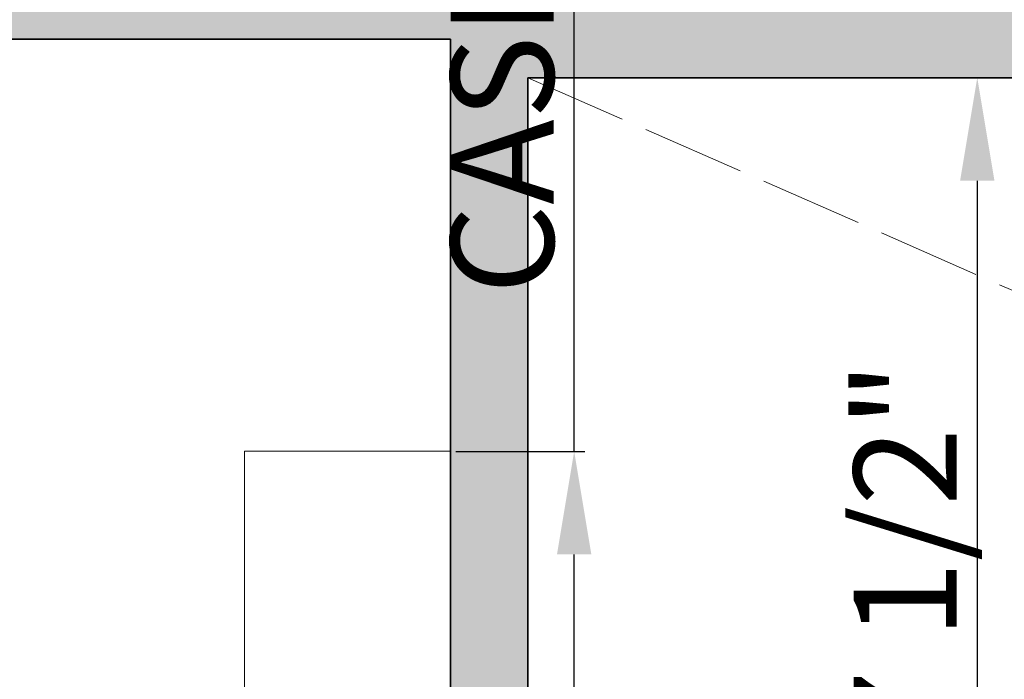
# Model space of a CAD drawing. Units: inches. Extents: x 2083 to 3317, y 1141 to 2115.
# Tile 87 of 256: x 2486 to 2600, y 1342 to 1419. Entities that reach past the tile are written whole.
import ezdxf

# ---------------------------------------------------------------- set-up
doc = ezdxf.new("R2010")
doc.units = ezdxf.units.IN
doc.linetypes.add('ACAD_ISO02W100', pattern=[15, 12, -3])
for name, color, linetype, lineweight in [('A-ANNO-DIMS', 2, 'Continuous', 18), ('A-FLOR-CASE', 8, 'Continuous', 18), ('A-FLOR-OPEN', 8, 'ACAD_ISO02W100', 13), ('A-WALL', 7, 'Continuous', 35)]:
    doc.layers.add(name, color=color, linetype=linetype, lineweight=lineweight)
doc.layers.add('A-WALL-PATT', color=251, linetype='Continuous', lineweight=13, true_color=0x636466)
doc.styles.get("Standard").update_dxf_attribs({"font": 'arial.ttf'})
doc.dimstyles.new('ISO-25', dxfattribs={"dimtxt": 12, "dimasz": 12, "dimexe": 1.25, "dimexo": 0.625, "dimtad": 1, "dimlunit": 3, "dimtxsty": 'Standard', "dimcen": 2.5, "dimadec": 0, "dimazin": 0, "dimtfac": 1, "dimtmove": 0, "dimatfit": 3, "dimfxl": 1, "dimarcsym": 0})

# ---------------------------------------------------------------- blocks, each defined once
blk = doc.blocks.new('CASEWORK-96X24')
for q in [(0, 0), (24, 96)]:
    blk.add_line((0, 96), q)
blk = doc.blocks.new('*D24')
at = {"layer": 'A-ANNO-DIMS', "color": 0, "lineweight": -2, "transparency": 16777216}
for p, q in [((2550.36, 1368.26), (2550.36, 1556.98)), ((2536.58, 1368.26), (2551.61, 1368.26)), ((2550.36, 1284.26), (2550.36, 1356.26)), ((2536.58, 1272.26), (2551.61, 1272.26))]:
    blk.add_line(p, q, dxfattribs=at)
at = {"layer": 'A-ANNO-DIMS', "color": 0, "transparency": 16777216}
for points in [[(2548.36, 1356.26), (2552.36, 1356.26), (2550.36, 1368.26)], [(2548.36, 1284.26), (2552.36, 1284.26), (2550.36, 1272.26)]]:
    blk.add_solid(points, dxfattribs=at)
at = {"layer": 'Defpoints', "color": 0, "transparency": 16777216}
for p in [(2535.96, 1368.26), (2550.36, 1368.26), (2535.96, 1272.26)]:
    blk.add_point(p, dxfattribs=at)
at = {"layer": 'A-ANNO-DIMS', "color": 0, "transparency": 16777216, "insert": (2543.53, 1468.62), "char_height": 12, "attachment_point": 5, "rotation": 90}
blk.add_mtext('CASEWORK 8\'-0" TYP.', dxfattribs=at)
blk = doc.blocks.new('*D67')
at = {"layer": 'A-ANNO-DIMS', "color": 0, "lineweight": -2, "transparency": 16777216}
for p, q in [((2545.58, 1411.76), (2598.56, 1411.76)), ((2597.31, 1399.76), (2597.31, 1284.26)), ((2545.58, 1272.26), (2598.56, 1272.26))]:
    blk.add_line(p, q, dxfattribs=at)
at = {"layer": 'A-ANNO-DIMS', "color": 0, "transparency": 16777216}
for points in [[(2595.31, 1399.76), (2599.31, 1399.76), (2597.31, 1411.76)], [(2595.31, 1284.26), (2599.31, 1284.26), (2597.31, 1272.26)]]:
    blk.add_solid(points, dxfattribs=at)
at = {"layer": 'Defpoints', "color": 0, "transparency": 16777216}
for p in [(2544.96, 1411.76), (2544.96, 1272.26), (2597.31, 1272.26)]:
    blk.add_point(p, dxfattribs=at)
at = {"layer": 'A-ANNO-DIMS', "color": 0, "transparency": 16777216, "insert": (2590.48, 1342.01), "char_height": 12, "attachment_point": 5, "rotation": 90}
blk.add_mtext('11\'-7 1/2"', dxfattribs=at)

msp = doc.modelspace()

# ---------------------------------------------------------------- hatches: boundary and pattern name
at = {"layer": 'A-WALL-PATT'}
h = msp.add_hatch(color=256, dxfattribs=at)
h.dxf.hatch_style = 1
h.paths.add_polyline_path([(3126.96, 2020.761), (2748.96, 2020.761), (2604.96, 2020.761), (2226.96, 2020.761), (2226.96, 1702.761), (2466.96, 1702.761), (2466.96, 1582.761), (2418.96, 1582.761), (2418.96, 1477.761), (2226.96, 1477.761), (2226.96, 1263.261), (2544.96, 1263.261), (2544.96, 1411.761), (2604.96, 1411.761), (2685.96, 1411.761), (2685.96, 1420.761), (2604.96, 1420.761), (2604.96, 1573.761), (2604.96, 1702.761), (2604.96, 2011.761), (2748.96, 2011.761), (2748.96, 1702.761), (2862.96, 1702.761), (2862.96, 1621.761), (2871.96, 1621.761), (2871.96, 1702.761), (2883.96, 1702.761), (2883.96, 1706.939, -0.0264593), (2883.96, 1711.761), (2757.96, 1711.761), (2757.96, 1807.761), (2787.96, 1807.761), (2787.96, 1812.261), (2757.96, 1812.261), (2757.96, 2011.761), (2877.96, 2011.761), (2877.96, 1812.261), (2847.96, 1812.261), (2847.96, 1807.761), (2889.836, 1807.761), (2889.836, 1812.261), (2882.46, 1812.261), (2882.46, 2011.761), (3117.96, 2011.761), (3117.96, 1812.261), (2937.836, 1812.261), (2937.836, 1807.761), (2995.71, 1807.761), (2995.71, 1796.118), (3000.21, 1796.118), (3000.21, 1807.761), (3117.96, 1807.761), (3117.96, 1711.761), (3000.21, 1711.761), (3000.21, 1760.118), (2998.573, 1760.118, -0.020711), (2995.71, 1760.118), (2995.71, 1711.761), (2931.96, 1711.761), (2931.96, 1702.761), (3126.96, 1702.761)])
h.paths.add_polyline_path([(2471.46, 2011.761), (2471.46, 1810.011), (2462.717, 1810.011), (2462.717, 1805.511), (2505.96, 1805.511), (2505.96, 1810.011), (2475.96, 1810.011), (2475.96, 2011.761), (2595.96, 2011.761), (2595.96, 1810.011), (2565.96, 1810.011), (2565.96, 1805.511), (2595.96, 1805.511), (2595.96, 1711.761), (2235.96, 1711.761), (2235.96, 1805.511), (2353.71, 1805.511), (2353.71, 1796.054), (2358.21, 1796.054), (2358.21, 1805.511), (2414.717, 1805.511), (2414.717, 1810.011), (2235.96, 1810.011), (2235.96, 2011.761)], flags=16)
h.paths.add_polyline_path([(2270.205, 1994.61), (2270.205, 1970.61), (2246.205, 1970.61), (2246.205, 1994.61)], flags=0)
edge = h.paths.add_edge_path(flags=0)
edge.add_ellipse((2332.027, 1899.798), major_axis=(-3.043, 3.043), ratio=0.1682525, start_angle=-161.33217, end_angle=-156.30711, ccw=False)
edge.add_ellipse((2333.082, 1898.744), major_axis=(-1.055, 1.055), ratio=0.4535321, start_angle=-123.37102, end_angle=-94.15911)
edge = h.paths.add_edge_path(flags=0)
edge.add_ellipse((2332.027, 1968.876), major_axis=(3.043, 3.043), ratio=0.1682525, start_angle=18.66783, end_angle=23.69289)
edge.add_spline(control_points=[(2332.926, 1970.691), (2332.227, 1970.336), (2330.894, 1969.659), (2328.413, 1970.932), (2327.204, 1967.749), (2324.71, 1969.956), (2322.533, 1967.012), (2320.013, 1971.296), (2317.68, 1968.158), (2316.041, 1967.102), (2315.427, 1966.81)], knot_values=[0, 0, 0, 0, 2.2670587, 4.3245589, 6.6855835, 8.8786411, 11.121502, 14.300359, 17.7552837, 19.732645, 19.732645, 19.732645, 19.732645], degree=3, periodic=0)
edge.add_ellipse((2332.027, 1968.876), major_axis=(3.043, 3.043), ratio=0.1682525, start_angle=18.66783, end_angle=23.69289, ccw=False)
edge.add_ellipse((2333.082, 1969.931), major_axis=(1.055, 1.055), ratio=0.4535321, start_angle=56.62898, end_angle=85.84089, ccw=False)
edge = h.paths.add_edge_path(flags=0)
edge.add_spline(control_points=[(2296.428, 1967.988), (2293.628, 1965.336), (2287.704, 1959.727), (2299.744, 1949.996), (2294.533, 1935.669), (2290.573, 1920.604), (2293.394, 1909.974), (2296.185, 1904.967)], knot_values=[0.0991853, 0.0991853, 0.0991853, 0.0991853, 0.3453009, 0.6198217, 0.9826526, 1.3860932, 1.8105546, 1.8105546, 1.8105546, 1.8105546], degree=3, periodic=0)
edge.add_spline(control_points=[(2296.185, 1904.967), (2297.384, 1902.619), (2298.001, 1901.949), (2298.553, 1901.468)], knot_values=[0.0062457, 0.0062457, 0.0062457, 0.0062457, 0.0554759, 0.0554759, 0.0554759, 0.0554759], degree=3, periodic=0)
edge.add_spline(control_points=[(2298.553, 1901.468), (2297.259, 1900.923), (2295.225, 1900.232), (2293.06, 1900.614), (2292.101, 1900.788), (2292.09, 1900.791)], knot_values=[0.3128349, 0.3128349, 0.3128349, 0.3128349, 0.4017797, 0.4749867, 0.4759027, 0.4759027, 0.4759027, 0.4759027], degree=3, periodic=0)
edge.add_arc((2292.794, 1904.664), 3.937, 215.4209, 259.69818, ccw=False)
edge.add_spline(control_points=[(2289.585, 1902.382), (2289.477, 1902.535), (2289.368, 1902.688), (2289.261, 1902.841)], knot_values=[0.1028719, 0.1028719, 0.1028719, 0.1028719, 0.1168958, 0.1168958, 0.1168958, 0.1168958], degree=3, periodic=0)
edge.add_spline(control_points=[(2289.261, 1902.841), (2288.687, 1902.55), (2287.64, 1902.02), (2285.881, 1901.874), (2283.853, 1901.504), (2281.72, 1899.711), (2278.467, 1899.493), (2276.157, 1901.883), (2272.259, 1899.804), (2267.778, 1901.843), (2262.244, 1900.184), (2257.415, 1901.782), (2254.318, 1900.726), (2253.178, 1900.337)], knot_values=[0, 0, 0, 0, 1.9079767, 3.4771759, 5.261074, 7.9728515, 11.6802485, 13.7179214, 16.9395917, 22.789562, 27.5025027, 33.5952153, 37.1456181, 37.1456181, 37.1456181, 37.1456181], degree=3, periodic=0)
edge.add_line((2253.178, 1900.337), (2250.244, 1902.841))
edge.add_line((2250.244, 1902.841), (2250.244, 1965.833))
edge.add_line((2250.244, 1965.833), (2253.178, 1968.337))
edge.add_spline(control_points=[(2253.178, 1968.337), (2254.318, 1967.948), (2257.415, 1966.892), (2262.244, 1968.49), (2267.778, 1966.831), (2271.527, 1968.537), (2273.876, 1967.828), (2274.207, 1967.728)], knot_values=[0, 0, 0, 0, 0.0901802, 0.2449351, 0.3646438, 0.5132331, 0.5378548, 0.5378548, 0.5378548, 0.5378548], degree=3, periodic=0)
edge.add_arc((2274.353, 1963.793), 3.937, 72.05113, 92.12795, ccw=False)
edge.add_arc((2281.297, 1985.23), 18.596, 252.05113, 288.56572)
edge.add_arc((2292.317, 1956.029), 12.646, 71.02679, 113.77822, ccw=False)
edge = h.paths.add_edge_path(flags=0)
edge.add_spline(control_points=[(2274.899, 1951.856), (2275.066, 1951.617), (2275.233, 1951.377), (2275.398, 1951.136)], knot_values=[1.4099157, 1.4099157, 1.4099157, 1.4099157, 1.4315903, 1.4315903, 1.4315903, 1.4315903], degree=3, periodic=0)
edge.add_spline(control_points=[(2275.398, 1951.136), (2275.792, 1950.562), (2276.179, 1949.984), (2276.546, 1949.397)], knot_values=[1.3582378, 1.3582378, 1.3582378, 1.3582378, 1.4099157, 1.4099157, 1.4099157, 1.4099157], degree=3, periodic=0)
edge.add_line((2276.546, 1949.397), (2277.437, 1947.862))
edge.add_spline(control_points=[(2277.437, 1947.862), (2276.304, 1945.673), (2274.64, 1942.427), (2274.632, 1938.094), (2272.799, 1930.852), (2274.356, 1943.897), (2275.948, 1947.923), (2276.546, 1949.397)], knot_values=[0.0056315, 0.0056315, 0.0056315, 0.0056315, 0.1860139, 0.2660015, 0.3570872, 0.5963902, 0.7397317, 0.7397317, 0.7397317, 0.7397317], degree=3, periodic=0)
edge.add_spline(control_points=[(2276.546, 1949.397), (2276.179, 1949.984), (2275.792, 1950.562), (2275.398, 1951.136)], knot_values=[1.3582378, 1.3582378, 1.3582378, 1.3582378, 1.4099157, 1.4099157, 1.4099157, 1.4099157], degree=3, periodic=0)
edge.add_spline(control_points=[(2275.398, 1951.136), (2274.943, 1950.08), (2274.208, 1948.025), (2273.935, 1944.851), (2272.469, 1937.627), (2273.466, 1945.696), (2274.701, 1951.059), (2274.899, 1951.856)], knot_values=[0.1043639, 0.1043639, 0.1043639, 0.1043639, 0.1896363, 0.2696239, 0.3607096, 0.6000126, 0.6446217, 0.6446217, 0.6446217, 0.6446217], degree=3, periodic=0)
h.paths.add_polyline_path([(2269.168, 1963.128, -0.3575267), (2268.171, 1960.976, -0.0925607), (2268.171, 1939.436, -0.3575267), (2269.168, 1937.285, -0.3575267), (2267.016, 1938.282, -0.1647847), (2254.686, 1938.282, -0.3575267), (2252.534, 1937.285, -0.3575267), (2253.531, 1939.436, -0.0925607), (2253.531, 1960.976, -0.3575267), (2252.534, 1963.128, -0.3575267), (2254.686, 1962.131, -0.1647847), (2267.016, 1962.131, -0.3575267)], flags=0)
h.paths.add_polyline_path([(2248.874, 1967.802), (2248.874, 1957.028), (2249.458, 1957.028), (2249.458, 1911.647), (2248.874, 1911.647), (2248.874, 1900.873), (2246.512, 1900.873, 0.1973271), (2244.15, 1902.457), (2244.15, 1966.218, 0.1973271), (2246.512, 1967.802)], flags=0)
h.paths.add_polyline_path([(2269.168, 1931.389, -0.3575267), (2268.171, 1929.238, -0.0925607), (2268.171, 1907.698, -0.3575267), (2269.168, 1905.547, -0.3575267), (2267.016, 1906.544, -0.1647847), (2254.686, 1906.544, -0.3575267), (2252.534, 1905.547, -0.3575267), (2253.531, 1907.698, -0.0925607), (2253.531, 1929.238, -0.3575267), (2252.534, 1931.389, -0.3575267), (2254.686, 1930.392, -0.1647847), (2267.016, 1930.392, -0.3575267)], flags=0)
edge = h.paths.add_edge_path(flags=0)
edge.add_spline(control_points=[(2276.197, 1906.724), (2276.168, 1909.029), (2276.114, 1913.372), (2270.598, 1924.925), (2273.905, 1919.013), (2275.922, 1916.262), (2275.475, 1912.402), (2277.258, 1910.381), (2276.696, 1908.225), (2276.646, 1906.813), (2276.618, 1906.008)], knot_values=[0, 0, 0, 0, 8.6102597, 16.2212739, 18.8430575, 23.8048978, 27.4408283, 29.3561016, 31.2034776, 33.6506866, 33.6506866, 33.6506866, 33.6506866], degree=3, periodic=0)
edge.add_spline(control_points=[(2276.618, 1906.008), (2276.623, 1905.624), (2276.498, 1904.629), (2275.442, 1903.855), (2274.937, 1903.08), (2274.859, 1902.841)], knot_values=[0.1564884, 0.1564884, 0.1564884, 0.1564884, 0.1843975, 0.2313765, 0.2505985, 0.2505985, 0.2505985, 0.2505985], degree=3, periodic=0)
edge.add_line((2274.859, 1902.841), (2276.506, 1902.841))
edge.add_spline(control_points=[(2276.506, 1902.841), (2276.788, 1903.085), (2277.665, 1904.125), (2278.25, 1904.341), (2277.654, 1908.527), (2278.156, 1906.228), (2278.1, 1905.286), (2278.847, 1904.069), (2277.857, 1903.415), (2277.874, 1902.991), (2277.904, 1902.841)], knot_values=[0.0595743, 0.0595743, 0.0595743, 0.0595743, 0.0807529, 0.1037415, 0.1697201, 0.1760361, 0.2071372, 0.2404744, 0.2623409, 0.2736605, 0.2736605, 0.2736605, 0.2736605], degree=3, periodic=0)
edge.add_line((2277.904, 1902.841), (2280.03, 1902.841))
edge.add_spline(control_points=[(2280.03, 1902.841), (2279.888, 1903.088), (2279.499, 1903.982), (2280.152, 1905.939), (2278.104, 1909.658), (2279.762, 1907.185), (2280.328, 1904.875), (2280.485, 1903.49), (2281.463, 1903.249), (2281.758, 1902.936), (2281.834, 1902.841)], knot_values=[0.013856, 0.013856, 0.013856, 0.013856, 0.0348738, 0.0888667, 0.1078792, 0.1267378, 0.158714, 0.1937575, 0.2174868, 0.2267221, 0.2267221, 0.2267221, 0.2267221], degree=3, periodic=0)
edge.add_spline(control_points=[(2281.834, 1902.841), (2281.788, 1902.827), (2281.647, 1902.783), (2281.396, 1902.859), (2281.088, 1902.985), (2280.721, 1903.061), (2280.333, 1903.026), (2280.125, 1902.899), (2280.03, 1902.841)], knot_values=[0, 0, 0, 0, 0.1441304, 0.435517, 0.7492759, 1.1530457, 1.5483707, 1.878348, 1.878348, 1.878348, 1.878348], degree=3, periodic=0)
edge.add_line((2280.03, 1902.841), (2277.904, 1902.841))
edge.add_spline(control_points=[(2277.904, 1902.841), (2277.893, 1902.796), (2277.865, 1902.68), (2277.607, 1902.687), (2277.274, 1902.801), (2276.838, 1902.62), (2276.584, 1902.789), (2276.506, 1902.841)], knot_values=[0, 0, 0, 0, 0.1271885, 0.3261988, 0.6280094, 1.2435704, 1.5153306, 1.5153306, 1.5153306, 1.5153306], degree=3, periodic=0)
edge.add_line((2276.506, 1902.841), (2274.859, 1902.841))
edge.add_spline(control_points=[(2274.859, 1902.841), (2274.814, 1902.899), (2274.725, 1903.013), (2274.493, 1903.119), (2274.244, 1902.961), (2273.937, 1903.185), (2273.614, 1902.983), (2273.408, 1902.883), (2273.322, 1902.841)], knot_values=[0, 0, 0, 0, 0.2184302, 0.4369566, 0.6879766, 0.9903786, 1.3983955, 1.6918498, 1.6918498, 1.6918498, 1.6918498], degree=3, periodic=0)
edge.add_spline(control_points=[(2273.322, 1902.841), (2273.617, 1903.446), (2274.274, 1904.538), (2276.027, 1904.574), (2276.207, 1906.584), (2276.197, 1906.724)], knot_values=[0.0122268, 0.0122268, 0.0122268, 0.0122268, 0.0594721, 0.1062177, 0.134458, 0.134458, 0.134458, 0.134458], degree=3, periodic=0)
h.paths.add_polyline_path([(2270.776, 1897.79), (2270.776, 1873.79), (2246.776, 1873.79), (2246.776, 1897.79)], flags=0)
h.paths.add_polyline_path([(2353.71, 1760.005), (2353.71, 1760.054), (2358.21, 1760.054, -0.033729)], flags=0)
h.paths.add_polyline_path([(2321.819, 1737.529), (2341.995, 1737.529, -0.4142136), (2343.203, 1736.321), (2343.203, 1721.021, -0.4142136), (2341.995, 1719.813), (2321.819, 1719.813, -0.4142136), (2320.611, 1721.021), (2320.611, 1736.321, -0.4142136)], flags=0)
h.paths.add_polyline_path([(2324.235, 1736.321), (2339.579, 1736.321, -0.4142136), (2341.995, 1733.905), (2341.995, 1725.45, -0.4142136), (2339.579, 1723.034), (2333.681, 1723.034), (2333.845, 1722.045, -0.8706461), (2335.425, 1721.826, -0.767327), (2333.923, 1721.423), (2331.291, 1721.423, -0.767327), (2329.788, 1721.826, -0.8706461), (2331.368, 1722.045), (2331.533, 1723.034), (2324.235, 1723.034, -0.4142136), (2321.819, 1725.45), (2321.819, 1733.905, -0.4142136)], flags=0)
h.paths.add_polyline_path([(2570.484, 1928.615), (2589.684, 1928.615), (2590.169, 1928.615), (2590.169, 1904.993), (2570.484, 1904.993)], flags=0)
h.paths.add_polyline_path([(2574.447, 1927.264, -1), (2572.829, 1927.264, -1)], flags=0)
h.paths.add_polyline_path([(2573.09, 1926.941), (2573.925, 1927.776), (2574.148, 1927.553), (2573.313, 1926.718)], flags=0)
h.paths.add_polyline_path([(2578.779, 1919.73, -1), (2571.592, 1919.73, -1)], flags=0)
h.paths.add_polyline_path([(2578.385, 1919.73, -1), (2571.985, 1919.73, -1)], flags=0)
h.paths.add_polyline_path([(2331.596, 1729.476, -1), (2333.618, 1729.476, -1)], flags=0)
h.paths.add_polyline_path([(2578.034, 1927.264, -1), (2576.416, 1927.264, -1)], flags=0)
h.paths.add_polyline_path([(2576.689, 1927.531), (2576.912, 1927.754), (2577.747, 1926.919), (2577.524, 1926.696)], flags=0)
h.paths.add_polyline_path([(2578.139, 1909.86, -1), (2572.232, 1909.86, -1)], flags=0)
h.paths.add_polyline_path([(2577.745, 1909.86, -1), (2572.625, 1909.86, -1)], flags=0)
h.paths.add_polyline_path([(2583.798, 1927.264, -1), (2582.179, 1927.264, -1)], flags=0)
h.paths.add_polyline_path([(2582.719, 1927.754), (2583.554, 1926.919), (2583.331, 1926.696), (2582.496, 1927.531)], flags=0)
h.paths.add_polyline_path([(2582.496, 1927.531), (2582.719, 1927.754), (2583.554, 1926.919), (2583.331, 1926.696)], flags=0)
h.paths.add_polyline_path([(2587.739, 1920.53, -1), (2581.832, 1920.53, -1)], flags=0)
h.paths.add_polyline_path([(2587.345, 1920.53, -1), (2582.225, 1920.53, -1)], flags=0)
h.paths.add_polyline_path([(2587.385, 1927.264, -1), (2585.766, 1927.264, -1)], flags=0)
h.paths.add_polyline_path([(2586.082, 1926.98), (2586.917, 1927.815), (2587.14, 1927.593), (2586.305, 1926.758)], flags=0)
h.paths.add_polyline_path([(2588.379, 1910.66, -1), (2581.192, 1910.66, -1)], flags=0)
h.paths.add_polyline_path([(2587.985, 1910.66, -1), (2581.585, 1910.66, -1)], flags=0)
h.paths.add_polyline_path([(2417.168, 1729.478), (2437.344, 1729.478, -0.4142136), (2438.552, 1728.27), (2438.552, 1712.969, -0.4142136), (2437.344, 1711.761), (2417.168, 1711.761, -0.4142136), (2415.96, 1712.969), (2415.96, 1728.27, -0.4142136)], flags=0)
h.paths.add_polyline_path([(2419.584, 1728.27), (2434.928, 1728.27, -0.4142136), (2437.344, 1725.854), (2437.344, 1717.398, -0.4142136), (2434.928, 1714.983), (2429.029, 1714.983), (2429.194, 1713.994, -0.8706461), (2430.774, 1713.775, -0.767327), (2429.271, 1713.372), (2426.64, 1713.372, -0.767327), (2425.137, 1713.775, -0.8706461), (2426.717, 1713.994), (2426.882, 1714.983), (2419.584, 1714.983, -0.4142136), (2417.168, 1717.398), (2417.168, 1725.854, -0.4142136)], flags=0)
h.paths.add_polyline_path([(2419.584, 1728.27), (2434.928, 1728.27, -0.4142136), (2437.344, 1725.854), (2437.344, 1717.398, -0.4142136), (2434.928, 1714.983), (2429.029, 1714.983), (2428.358, 1719.009), (2427.553, 1719.009), (2426.882, 1714.983), (2419.584, 1714.983, -0.4142136), (2417.168, 1717.398), (2417.168, 1725.854, -0.4142136)], flags=0)
h.paths.add_polyline_path([(2426.944, 1721.425, -1), (2428.967, 1721.425, -1)], flags=0)
h.paths.add_polyline_path([(2475.96, 1702.761), (2595.96, 1702.761), (2595.96, 1582.761), (2475.96, 1582.761)], flags=16)
h.paths.add_polyline_path([(2427.96, 1573.761), (2595.96, 1573.761), (2595.96, 1468.761), (2595.96, 1420.761), (2384.46, 1420.761), (2384.46, 1468.761), (2427.96, 1468.761)], flags=16)
h.paths.add_polyline_path([(2379.96, 1468.761), (2379.96, 1420.761), (2235.96, 1420.761), (2235.96, 1468.761)], flags=16)
h.paths.add_polyline_path([(2317.816, 1466.696), (2337.992, 1466.696, -0.4142136), (2339.2, 1465.488), (2339.2, 1450.187, -0.4142136), (2337.992, 1448.979), (2317.816, 1448.979, -0.4142136), (2316.608, 1450.187), (2316.608, 1465.488, -0.4142136)], flags=0)
h.paths.add_polyline_path([(2320.232, 1465.488), (2335.576, 1465.488, -0.4142136), (2337.992, 1463.072), (2337.992, 1454.616, -0.4142136), (2335.576, 1452.2), (2329.677, 1452.2), (2329.842, 1451.212, -0.8706461), (2331.422, 1450.992, -0.767327), (2329.92, 1450.59), (2327.288, 1450.59, -0.767327), (2325.785, 1450.992, -0.8706461), (2327.365, 1451.212), (2327.53, 1452.2), (2320.232, 1452.2, -0.4142136), (2317.816, 1454.616), (2317.816, 1463.072, -0.4142136)], flags=0)
h.paths.add_polyline_path([(2320.232, 1465.488), (2335.576, 1465.488, -0.4142136), (2337.992, 1463.072), (2337.992, 1454.616, -0.4142136), (2335.576, 1452.2), (2329.677, 1452.2), (2329.006, 1456.227), (2328.201, 1456.227), (2327.53, 1452.2), (2320.232, 1452.2, -0.4142136), (2317.816, 1454.616), (2317.816, 1463.072, -0.4142136)], flags=0)
h.paths.add_polyline_path([(2327.593, 1458.643, -1), (2329.615, 1458.643, -1)], flags=0)
h.paths.add_polyline_path([(2244.412, 1433.34), (2241.921, 1433.34, -0.4142136), (2240.018, 1435.244), (2240.018, 1440.953, -0.4142105), (2241.921, 1442.856), (2244.412, 1442.856, -1.9764724)], flags=0)
h.paths.add_polyline_path([(2245.357, 1434.398, -0.4142136), (2245.357, 1441.799, -2.1440985)], flags=0)
h.paths.add_polyline_path([(2535.96, 1416.261), (2535.96, 1272.261), (2235.96, 1272.261), (2235.96, 1416.261)], flags=16)
h.paths.add_polyline_path([(2260.12, 1384.293), (2260.12, 1362.039), (2237.865, 1362.039), (2237.865, 1384.293)], flags=0)
edge = h.paths.add_edge_path(flags=0)
edge.add_line((2318.252, 1362.093), (2318.146, 1362.001))
edge.add_ellipse((2317.445, 1360.431), major_axis=(2.822, 2.822), ratio=0.1682525, start_angle=18.66783, end_angle=20.94813, ccw=False)
edge.add_ellipse((2318.423, 1361.409), major_axis=(0.978, 0.978), ratio=0.4535321, start_angle=56.62898, end_angle=70.2262, ccw=False)
edge = h.paths.add_edge_path(flags=0)
edge.add_line((2319.107, 1295.571), (2319.015, 1295.677))
edge.add_ellipse((2317.445, 1296.378), major_axis=(-2.822, 2.822), ratio=0.1682525, start_angle=-161.33217, end_angle=-159.05187, ccw=False)
edge.add_ellipse((2318.423, 1295.4), major_axis=(-0.978, 0.978), ratio=0.4535321, start_angle=-123.37102, end_angle=-109.7738)
edge = h.paths.add_edge_path(flags=0)
edge.add_spline(control_points=[(2284.21, 1301.17), (2284.581, 1300.445), (2284.891, 1299.892), (2285.16, 1299.461)], knot_values=[0.0390658, 0.0390658, 0.0390658, 0.0390658, 0.0554759, 0.0554759, 0.0554759, 0.0554759], degree=3, periodic=0)
edge.add_line((2285.16, 1299.461), (2284.21, 1301.17))
edge = h.paths.add_edge_path(flags=0)
edge.add_line((2280.412, 1297.298), (2283.37, 1297.036))
edge.add_line((2283.37, 1297.036), (2286.406, 1297.926))
edge.add_spline(control_points=[(2286.406, 1297.926), (2285.305, 1297.463), (2284.345, 1297.129), (2283.37, 1297.036)], knot_values=[0.3943688, 0.3943688, 0.3943688, 0.3943688, 0.4759027, 0.4759027, 0.4759027, 0.4759027], degree=3, periodic=0)
edge.add_spline(control_points=[(2283.37, 1297.036), (2283.281, 1297.028), (2282.316, 1296.957), (2281.313, 1297.134), (2280.423, 1297.296), (2280.412, 1297.298)], knot_values=[0.3128349, 0.3128349, 0.3128349, 0.3128349, 0.3202458, 0.3934528, 0.3943688, 0.3943688, 0.3943688, 0.3943688], degree=3, periodic=0)
edge = h.paths.add_edge_path(flags=0)
edge.add_line((2284.436, 1359.607), (2280.446, 1355.328))
edge.add_line((2280.446, 1355.328), (2279.58, 1351.018))
edge.add_line((2279.58, 1351.018), (2282.413, 1346.58))
edge.add_spline(control_points=[(2282.413, 1346.58), (2283.153, 1345.589), (2284.253, 1344.029), (2284.801, 1342.387), (2284.935, 1341.806)], knot_values=[1.2400982, 1.2400982, 1.2400982, 1.2400982, 1.3328922, 1.3827123, 1.3827123, 1.3827123, 1.3827123], degree=3, periodic=0)
edge.add_spline(control_points=[(2284.935, 1341.806), (2285.319, 1340.141), (2285.233, 1338.409), (2284.91, 1336.654)], knot_values=[1.0974841, 1.0974841, 1.0974841, 1.0974841, 1.2400982, 1.2400982, 1.2400982, 1.2400982], degree=3, periodic=0)
edge.add_spline(control_points=[(2284.91, 1336.654), (2284.587, 1334.899), (2284.027, 1333.12), (2283.463, 1331.361)], knot_values=[0.9548699, 0.9548699, 0.9548699, 0.9548699, 1.0974841, 1.0974841, 1.0974841, 1.0974841], degree=3, periodic=0)
edge.add_line((2283.463, 1331.361), (2281.89, 1326.153))
edge.add_line((2281.89, 1326.153), (2280.756, 1321.056))
edge.add_line((2280.756, 1321.056), (2280.299, 1316.002))
edge.add_line((2280.299, 1316.002), (2280.716, 1310.95))
edge.add_line((2280.716, 1310.95), (2282.028, 1305.972))
edge.add_line((2282.028, 1305.972), (2284.21, 1301.17))
edge.add_spline(control_points=[(2284.21, 1301.17), (2283.341, 1302.73), (2282.612, 1304.336), (2282.028, 1305.972)], knot_values=[0.0991853, 0.0991853, 0.0991853, 0.0991853, 0.2417994, 0.2417994, 0.2417994, 0.2417994], degree=3, periodic=0)
edge.add_spline(control_points=[(2282.028, 1305.972), (2281.444, 1307.608), (2281.005, 1309.273), (2280.716, 1310.95)], knot_values=[0.2417994, 0.2417994, 0.2417994, 0.2417994, 0.3844135, 0.3844135, 0.3844135, 0.3844135], degree=3, periodic=0)
edge.add_spline(control_points=[(2280.716, 1310.95), (2280.433, 1312.588), (2280.289, 1314.277), (2280.299, 1315.962), (2280.299, 1316.002)], knot_values=[0.3844135, 0.3844135, 0.3844135, 0.3844135, 0.5236467, 0.5270276, 0.5270276, 0.5270276, 0.5270276], degree=3, periodic=0)
edge.add_spline(control_points=[(2280.299, 1316.002), (2280.312, 1317.687), (2280.478, 1319.368), (2280.756, 1321.056)], knot_values=[0.5270276, 0.5270276, 0.5270276, 0.5270276, 0.6696417, 0.6696417, 0.6696417, 0.6696417], degree=3, periodic=0)
edge.add_spline(control_points=[(2280.756, 1321.056), (2281.035, 1322.744), (2281.426, 1324.44), (2281.89, 1326.153)], knot_values=[0.6696417, 0.6696417, 0.6696417, 0.6696417, 0.8122558, 0.8122558, 0.8122558, 0.8122558], degree=3, periodic=0)
edge.add_spline(control_points=[(2281.89, 1326.153), (2282.264, 1327.533), (2282.788, 1329.262), (2283.353, 1331.018), (2283.463, 1331.361)], knot_values=[0.8122558, 0.8122558, 0.8122558, 0.8122558, 0.9270873, 0.9548699, 0.9548699, 0.9548699, 0.9548699], degree=3, periodic=0)
edge.add_line((2283.463, 1331.361), (2284.91, 1336.654))
edge.add_line((2284.91, 1336.654), (2284.935, 1341.806))
edge.add_line((2284.935, 1341.806), (2282.413, 1346.58))
edge.add_spline(control_points=[(2282.413, 1346.58), (2281.275, 1348.104), (2280.078, 1349.57), (2279.58, 1351.018)], knot_values=[1.3827123, 1.3827123, 1.3827123, 1.3827123, 1.5253264, 1.5253264, 1.5253264, 1.5253264], degree=3, periodic=0)
edge.add_spline(control_points=[(2279.58, 1351.018), (2279.443, 1351.415), (2279.136, 1352.857), (2279.735, 1354.29), (2280.446, 1355.328)], knot_values=[1.5253264, 1.5253264, 1.5253264, 1.5253264, 1.564439, 1.6679405, 1.6679405, 1.6679405, 1.6679405], degree=3, periodic=0)
edge.add_spline(control_points=[(2280.446, 1355.328), (2281.426, 1356.758), (2282.931, 1358.183), (2284.436, 1359.607)], knot_values=[1.6679405, 1.6679405, 1.6679405, 1.6679405, 1.8105546, 1.8105546, 1.8105546, 1.8105546], degree=3, periodic=0)
edge.add_arc((2280.623, 1348.518), 11.726, 71.02679, 113.77822)
edge.add_arc((2270.405, 1375.595), 17.244, 252.05113, 288.56572, ccw=False)
edge.add_arc((2263.966, 1355.718), 3.651, 72.05113, 92.12795)
edge.add_arc((2263.966, 1355.718), 3.651, 92.12795, 177.98513)
edge.add_spline(control_points=[(2260.318, 1355.846), (2260.26, 1354.221), (2260.551, 1350.187), (2262.999, 1346.766), (2264.473, 1344.649)], knot_values=[1.4315903, 1.4315903, 1.4315903, 1.4315903, 1.5641438, 1.7706953, 1.7706953, 1.7706953, 1.7706953], degree=3, periodic=0)
edge.add_line((2264.473, 1344.649), (2264.936, 1343.983))
edge.add_spline(control_points=[(2263.801, 1340.248), (2263.843, 1340.514), (2264.067, 1341.756), (2264.513, 1343.002), (2264.935, 1343.981)], knot_values=[0.5365702, 0.5365702, 0.5365702, 0.5365702, 0.5593494, 0.6446217, 0.6446217, 0.6446217, 0.6446217], degree=3, periodic=0)
edge.add_spline(control_points=[(2264.935, 1343.981), (2265.118, 1343.715), (2265.299, 1343.448), (2265.477, 1343.179)], knot_values=[1.3840767, 1.3840767, 1.3840767, 1.3840767, 1.4099157, 1.4099157, 1.4099157, 1.4099157], degree=3, periodic=0)
edge.add_spline(control_points=[(2265.477, 1343.179), (2265.655, 1342.911), (2265.829, 1342.641), (2265.999, 1342.369)], knot_values=[1.3582378, 1.3582378, 1.3582378, 1.3582378, 1.3840767, 1.3840767, 1.3840767, 1.3840767], degree=3, periodic=0)
edge.add_line((2265.999, 1342.369), (2266.826, 1340.946))
edge.add_spline(control_points=[(2266.826, 1340.946), (2268.894, 1337.09), (2271.398, 1325.843), (2270.516, 1310.569), (2275.919, 1301.861), (2277.79, 1299.199)], knot_values=[0.1168958, 0.1168958, 0.1168958, 0.1168958, 0.4729873, 1.0509689, 1.3137934, 1.3137934, 1.3137934, 1.3137934], degree=3, periodic=0)
edge.add_spline(control_points=[(2277.79, 1299.199), (2277.839, 1299.128), (2277.889, 1299.057), (2277.94, 1298.987)], knot_values=[0.1098839, 0.1098839, 0.1098839, 0.1098839, 0.1168958, 0.1168958, 0.1168958, 0.1168958], degree=3, periodic=0)
edge.add_line((2277.94, 1298.987), (2277.789, 1299.199))
edge.add_spline(control_points=[(2277.789, 1299.199), (2277.257, 1298.929), (2276.286, 1298.438), (2275.039, 1298.334), (2274.383, 1298.239), (2274.215, 1298.209)], knot_values=[33.1218702, 33.1218702, 33.1218702, 33.1218702, 35.0290557, 36.5982549, 37.1448269, 37.1448269, 37.1448269, 37.1448269], degree=3, periodic=0)
edge.add_line((2274.215, 1298.209), (2273.073, 1297.893))
edge.add_spline(control_points=[(2273.073, 1297.893), (2272.323, 1297.58), (2271.039, 1296.511), (2269.248, 1296.226), (2268.423, 1296.375)], knot_values=[26.5325843, 26.5325843, 26.5325843, 26.5325843, 29.198919, 31.8391012, 31.8391012, 31.8391012, 31.8391012], degree=3, periodic=0)
edge.add_line((2268.423, 1296.375), (2263.879, 1297.458))
edge.add_spline(control_points=[(2263.879, 1297.458), (2263.556, 1297.359), (2261.86, 1296.839), (2260.239, 1297.282), (2258.933, 1297.516)], knot_values=[15.9195506, 15.9195506, 15.9195506, 15.9195506, 16.9395917, 21.2260675, 21.2260675, 21.2260675, 21.2260675], degree=3, periodic=0)
edge.add_line((2258.933, 1297.516), (2254.055, 1297.329))
edge.add_spline(control_points=[(2254.055, 1297.329), (2253.756, 1297.296), (2252.114, 1297.165), (2250.462, 1297.544), (2249.13, 1297.668)], knot_values=[5.3065169, 5.3065169, 5.3065169, 5.3065169, 6.2764352, 10.6130337, 10.6130337, 10.6130337, 10.6130337], degree=3, periodic=0)
edge.add_line((2249.13, 1297.668), (2244.332, 1296.878))
edge.add_line((2244.332, 1296.878), (2241.611, 1299.199))
edge.add_line((2241.611, 1299.199), (2241.611, 1357.609))
edge.add_line((2241.611, 1357.609), (2244.332, 1359.931))
edge.add_line((2244.332, 1359.931), (2252.729, 1359.543))
edge.add_spline(control_points=[(2252.729, 1359.543), (2252.871, 1359.546), (2253.306, 1359.548), (2253.74, 1359.514), (2254.032, 1359.482)], knot_values=[0.233291, 0.233291, 0.233291, 0.233291, 0.2449351, 0.2689274, 0.2689274, 0.2689274, 0.2689274], degree=3, periodic=0)
edge.add_line((2254.032, 1359.482), (2259.587, 1359.416))
edge.add_spline(control_points=[(2259.587, 1359.416), (2260.677, 1359.629), (2262.073, 1359.897), (2263.524, 1359.459), (2263.83, 1359.366)], knot_values=[0.4225164, 0.4225164, 0.4225164, 0.4225164, 0.5132331, 0.5378548, 0.5378548, 0.5378548, 0.5378548], degree=3, periodic=0)
edge.add_arc((2263.966, 1355.718), 3.651, 72.05113, 92.12795, ccw=False)
edge.add_arc((2270.405, 1375.595), 17.244, 252.05113, 288.56572)
edge.add_arc((2280.623, 1348.518), 11.726, 71.02679, 113.77822, ccw=False)
h.paths.add_polyline_path([(2240.341, 1359.435), (2240.341, 1349.444), (2240.882, 1349.444), (2240.882, 1307.365), (2240.341, 1307.365), (2240.341, 1297.374), (2238.15, 1297.374, 0.1973271), (2235.96, 1298.843), (2235.96, 1357.966, 0.1973271), (2238.15, 1359.435)], flags=0)
h.paths.add_polyline_path([(2259.158, 1355.101, -0.3575267), (2258.233, 1353.106, -0.0925607), (2258.233, 1333.133, -0.3575267), (2259.158, 1331.138, -0.3575267), (2257.163, 1332.062, -0.1647847), (2245.729, 1332.062, -0.3575267), (2243.735, 1331.138, -0.3575267), (2244.659, 1333.133, -0.0925607), (2244.659, 1353.106, -0.3575267), (2243.735, 1355.101, -0.3575267), (2245.729, 1354.176, -0.1647847), (2257.163, 1354.176, -0.3575267)], flags=0)
edge = h.paths.add_edge_path(flags=0)
edge.add_line((2265.999, 1342.369), (2266.826, 1340.946))
edge.add_line((2266.826, 1340.946), (2265.308, 1337.814))
edge.add_line((2265.308, 1337.814), (2264.358, 1334.653))
edge.add_line((2264.358, 1334.653), (2264.262, 1333.8))
edge.add_spline(control_points=[(2264.262, 1333.8), (2264.208, 1333.187), (2264.162, 1332.366), (2264.007, 1331.414), (2263.969, 1331.202)], knot_values=[0.4644442, 0.4644442, 0.4644442, 0.4644442, 0.5166905, 0.5316081, 0.5316081, 0.5316081, 0.5316081], degree=3, periodic=0)
edge.add_spline(control_points=[(2263.969, 1331.202), (2263.775, 1330.119), (2263.424, 1328.791), (2263.257, 1328.531), (2263.234, 1328.515)], knot_values=[0.3726816, 0.3726816, 0.3726816, 0.3726816, 0.4488497, 0.4644442, 0.4644442, 0.4644442, 0.4644442], degree=3, periodic=0)
edge.add_spline(control_points=[(2263.234, 1328.515), (2263.096, 1328.42), (2263.131, 1329.301), (2263.275, 1330.616)], knot_values=[0.2809191, 0.2809191, 0.2809191, 0.2809191, 0.3726816, 0.3726816, 0.3726816, 0.3726816], degree=3, periodic=0)
edge.add_spline(control_points=[(2263.275, 1330.616), (2263.419, 1331.93), (2263.672, 1333.677), (2263.97, 1335.315)], knot_values=[0.1891566, 0.1891566, 0.1891566, 0.1891566, 0.2809191, 0.2809191, 0.2809191, 0.2809191], degree=3, periodic=0)
edge.add_spline(control_points=[(2263.97, 1335.315), (2264.1, 1336.032), (2264.419, 1337.622), (2264.755, 1338.864), (2264.947, 1339.491)], knot_values=[0.097394, 0.097394, 0.097394, 0.097394, 0.1375775, 0.1891566, 0.1891566, 0.1891566, 0.1891566], degree=3, periodic=0)
edge.add_spline(control_points=[(2264.947, 1339.491), (2265.29, 1340.606), (2265.644, 1341.494), (2265.999, 1342.369)], knot_values=[0.0056315, 0.0056315, 0.0056315, 0.0056315, 0.097394, 0.097394, 0.097394, 0.097394], degree=3, periodic=0)
h.paths.add_polyline_path([(2259.158, 1325.671, -0.3575267), (2258.233, 1323.676, -0.0925607), (2258.233, 1303.703, -0.3575267), (2259.158, 1301.708, -0.3575267), (2257.163, 1302.633, -0.1647847), (2245.729, 1302.633, -0.3575267), (2243.735, 1301.708, -0.3575267), (2244.659, 1303.703, -0.0925607), (2244.659, 1323.676, -0.3575267), (2243.735, 1325.671, -0.3575267), (2245.729, 1324.747, -0.1647847), (2257.163, 1324.747, -0.3575267)], flags=0)
edge = h.paths.add_edge_path(flags=0)
edge.add_spline(control_points=[(2261.709, 1317.311), (2261.679, 1317.418), (2261.762, 1317.389), (2262.491, 1316.09), (2262.962, 1315.301)], knot_values=[14.9558607, 14.9558607, 14.9558607, 14.9558607, 16.2212739, 18.6948259, 18.6948259, 18.6948259, 18.6948259], degree=3, periodic=0)
edge.add_spline(control_points=[(2262.962, 1315.301), (2262.99, 1315.254), (2263.702, 1314.067), (2264.349, 1313.127), (2264.73, 1312.164)], knot_values=[18.6948259, 18.6948259, 18.6948259, 18.6948259, 18.8430575, 22.433791, 22.433791, 22.433791, 22.433791], degree=3, periodic=0)
edge.add_spline(control_points=[(2264.73, 1312.164), (2264.876, 1311.796), (2265.177, 1310.77), (2265.143, 1309.559), (2265.248, 1308.824)], knot_values=[22.433791, 22.433791, 22.433791, 22.433791, 23.8048978, 26.1727562, 26.1727562, 26.1727562, 26.1727562], degree=3, periodic=0)
edge.add_line((2265.248, 1308.824), (2265.851, 1307.172))
edge.add_spline(control_points=[(2265.851, 1307.172), (2266.065, 1306.822), (2266.384, 1306.332), (2266.424, 1305.781), (2266.42, 1305.611)], knot_values=[28.0625624, 28.0625624, 28.0625624, 28.0625624, 29.3561016, 29.9117214, 29.9117214, 29.9117214, 29.9117214], degree=3, periodic=0)
edge.add_spline(control_points=[(2266.42, 1305.611), (2266.416, 1305.433), (2266.394, 1305.25), (2266.365, 1305.066)], knot_values=[29.9117214, 29.9117214, 29.9117214, 29.9117214, 30.4978371, 30.4978371, 30.4978371, 30.4978371], degree=3, periodic=0)
edge.add_line((2266.365, 1305.066), (2266.066, 1302.136))
edge.add_spline(control_points=[(2266.066, 1302.136), (2266.071, 1301.78), (2265.998, 1301.2), (2265.663, 1300.759), (2265.509, 1300.586)], knot_values=[0.1564884, 0.1564884, 0.1564884, 0.1564884, 0.1843975, 0.2035434, 0.2035434, 0.2035434, 0.2035434], degree=3, periodic=0)
edge.add_line((2265.509, 1300.586), (2264.435, 1299.199))
edge.add_line((2264.435, 1299.199), (2265.962, 1299.199))
edge.add_line((2265.962, 1299.199), (2267.336, 1301.175))
edge.add_line((2267.336, 1301.175), (2267.312, 1301.986))
edge.add_spline(control_points=[(2267.312, 1301.986), (2267.261, 1302.862), (2267.16, 1303.737), (2267.271, 1303.326)], knot_values=[0.1262286, 0.1262286, 0.1262286, 0.1262286, 0.1666174, 0.1666174, 0.1666174, 0.1666174], degree=3, periodic=0)
edge.add_spline(control_points=[(2267.271, 1303.326), (2267.28, 1303.294), (2267.31, 1303.175), (2267.373, 1302.884), (2267.406, 1302.683), (2267.418, 1302.601)], knot_values=[0.1666174, 0.1666174, 0.1666174, 0.1666174, 0.1697201, 0.1760361, 0.1807647, 0.1807647, 0.1807647, 0.1807647], degree=3, periodic=0)
edge.add_spline(control_points=[(2267.744, 1300.988), (2267.688, 1301.151), (2267.481, 1301.657), (2267.484, 1302.145), (2267.418, 1302.601)], knot_values=[0.1807647, 0.1807647, 0.1807647, 0.1807647, 0.1937665, 0.2201389, 0.2201389, 0.2201389, 0.2201389], degree=3, periodic=0)
edge.add_line((2267.418, 1302.601), (2267.744, 1300.988))
edge.add_spline(control_points=[(2267.744, 1300.988), (2267.832, 1300.732), (2267.932, 1300.31), (2267.555, 1299.975), (2267.429, 1299.829)], knot_values=[0.2201389, 0.2201389, 0.2201389, 0.2201389, 0.2404744, 0.2548903, 0.2548903, 0.2548903, 0.2548903], degree=3, periodic=0)
edge.add_line((2267.429, 1299.829), (2267.258, 1299.199))
edge.add_line((2267.258, 1299.199), (2269.23, 1299.199))
edge.add_spline(control_points=[(2269.23, 1299.199), (2269.099, 1299.429), (2268.843, 1300.016), (2269.012, 1300.916), (2268.947, 1301.661)], knot_values=[0.013856, 0.013856, 0.013856, 0.013856, 0.0348738, 0.0670726, 0.0670726, 0.0670726, 0.0670726], degree=3, periodic=0)
edge.add_line((2268.947, 1301.661), (2268.432, 1303.603))
edge.add_spline(control_points=[(2268.432, 1303.603), (2268.176, 1304.192), (2267.596, 1305.251), (2268.041, 1304.623), (2268.251, 1304.282)], knot_values=[0.0901547, 0.0901547, 0.0901547, 0.0901547, 0.1078792, 0.1202891, 0.1202891, 0.1202891, 0.1202891], degree=3, periodic=0)
edge.add_spline(control_points=[(2268.251, 1304.282), (2268.361, 1304.105), (2269.058, 1302.918), (2269.383, 1301.59), (2269.521, 1300.776), (2269.575, 1300.556)], knot_values=[0.1202891, 0.1202891, 0.1202891, 0.1202891, 0.1267378, 0.158714, 0.1735056, 0.1735056, 0.1735056, 0.1735056], degree=3, periodic=0)
edge.add_line((2269.575, 1300.556), (2270.686, 1299.421))
edge.add_spline(control_points=[(2270.686, 1299.421), (2270.767, 1299.357), (2270.838, 1299.281), (2270.903, 1299.199)], knot_values=[0.2181597, 0.2181597, 0.2181597, 0.2181597, 0.2267221, 0.2267221, 0.2267221, 0.2267221], degree=3, periodic=0)
edge.add_line((2270.937, 1299.193), (2270.903, 1299.199))
edge.add_spline(control_points=[(2270.903, 1299.199), (2270.86, 1299.186), (2270.73, 1299.146), (2270.496, 1299.216), (2270.272, 1299.308), (2270.121, 1299.348), (2270.063, 1299.36)], knot_values=[0.939174, 0.939174, 0.939174, 0.939174, 1.0833044, 1.3746911, 1.6884499, 1.878348, 1.878348, 1.878348, 1.878348], degree=3, periodic=0)
edge.add_line((2270.063, 1299.36), (2269.23, 1299.199))
edge.add_line((2269.23, 1299.199), (2267.258, 1299.199))
edge.add_spline(control_points=[(2267.258, 1299.199), (2267.248, 1299.157), (2267.223, 1299.05), (2266.984, 1299.057), (2266.809, 1299.116), (2266.677, 1299.109), (2266.637, 1299.105)], knot_values=[0.7576653, 0.7576653, 0.7576653, 0.7576653, 0.8848538, 1.0838641, 1.3856747, 1.5153306, 1.5153306, 1.5153306, 1.5153306], degree=3, periodic=0)
edge.add_spline(control_points=[(2266.637, 1299.105), (2266.485, 1299.089), (2266.236, 1299.017), (2266.035, 1299.151), (2265.962, 1299.199)], knot_values=[0, 0, 0, 0, 0.4859051, 0.7576653, 0.7576653, 0.7576653, 0.7576653], degree=3, periodic=0)
edge.add_line((2265.962, 1299.199), (2264.435, 1299.199))
edge.add_line((2264.435, 1299.199), (2263.858, 1299.367))
edge.add_spline(control_points=[(2263.858, 1299.367), (2263.819, 1299.371), (2263.78, 1299.386), (2263.74, 1299.402)], knot_values=[0.8459249, 0.8459249, 0.8459249, 0.8459249, 0.9786272, 0.9786272, 0.9786272, 0.9786272], degree=3, periodic=0)
edge.add_line((2263.722, 1299.396), (2263.01, 1299.199))
edge.add_spline(control_points=[(2263.01, 1299.199), (2263.246, 1299.683), (2263.506, 1300.128), (2263.873, 1300.408)], knot_values=[0.0122268, 0.0122268, 0.0122268, 0.0122268, 0.0529705, 0.0529705, 0.0529705, 0.0529705], degree=3, periodic=0)
edge.add_spline(control_points=[(2263.873, 1300.408), (2263.932, 1300.453), (2264.084, 1300.553), (2264.255, 1300.624), (2264.36, 1300.665)], knot_values=[0.0529705, 0.0529705, 0.0529705, 0.0529705, 0.0594721, 0.0690861, 0.0690861, 0.0690861, 0.0690861], degree=3, periodic=0)
edge.add_line((2264.36, 1300.665), (2265.142, 1301.078))
edge.add_line((2265.142, 1301.078), (2265.676, 1302.8))
edge.add_line((2265.676, 1302.8), (2265.541, 1305.704))
edge.add_line((2265.541, 1305.704), (2264.803, 1309.328))
edge.add_line((2264.803, 1309.328), (2263.041, 1314.092))
edge.add_spline(control_points=[(2263.041, 1314.092), (2262.384, 1315.671), (2261.796, 1316.998), (2261.709, 1317.311)], knot_values=[11.2168955, 11.2168955, 11.2168955, 11.2168955, 14.9558607, 14.9558607, 14.9558607, 14.9558607], degree=3, periodic=0)
h.paths.add_polyline_path([(2871.96, 1416.261), (2895.91, 1416.261), (2895.91, 1420.761), (2871.96, 1420.761), (2871.96, 1501.761), (2862.96, 1501.761), (2862.96, 1420.761), (2805.96, 1420.761), (2805.96, 1411.761), (2862.96, 1411.761), (2862.96, 1263.261), (3126.96, 1263.261), (3126.96, 1411.761), (3126.96, 1486.761), (2943.96, 1486.761), (2943.96, 1477.761), (2967.86, 1477.761), (2967.86, 1420.761), (2943.91, 1420.761), (2943.91, 1416.261), (3117.96, 1416.261), (3117.96, 1420.761), (2972.36, 1420.761), (2972.36, 1477.761), (3117.96, 1477.761), (3117.96, 1420.761), (3117.96, 1272.261), (2871.96, 1272.261)], flags=0)
h.paths.add_polyline_path([(2457.126, 1485.943), (2527.603, 1485.943), (2527.603, 1537.636), (2457.126, 1537.636)], flags=8)
h.paths.add_polyline_path([(2481.005, 1609.982), (2590.766, 1609.982), (2590.766, 1682.003), (2481.005, 1682.003)], flags=8)
h.paths.add_polyline_path([(2483.085, 1729.127), (2553.562, 1729.127), (2553.562, 1780.82), (2483.085, 1780.82)], flags=8)

# ---------------------------------------------------------------- linework, layer by layer
at = {"layer": 'A-FLOR-OPEN'}
msp.add_line((2544.96, 1411.761), (2862.96, 1272.261), dxfattribs=at)
at = {"layer": 'A-WALL'}
for p, q in [((2235.96, 1416.261), (2535.96, 1416.261)), ((2235.96, 1416.261), (2535.96, 1416.261)), ((2535.96, 1416.261), (2535.96, 1272.261)), ((2535.96, 1416.261), (2535.96, 1272.261)), ((2544.96, 1411.761), (2604.96, 1411.761)), ((2544.96, 1411.761), (2544.96, 1263.261))]:
    msp.add_line(p, q, dxfattribs=at)

# ---------------------------------------------------------------- block references
at = {"layer": 'A-FLOR-CASE'}
msp.add_blockref('CASEWORK-96X24', (2511.96, 1272.261), dxfattribs=at)

# ---------------------------------------------------------------- dimensions: what is measured, and where the dimension line sits
at = {"layer": 'A-ANNO-DIMS'}
dim = msp.add_linear_dim(base=(2550.36, 1368.261), p1=(2535.96, 1272.261), p2=(2535.96, 1368.261), angle=90, text='CASEWORK <> TYP.', dimstyle='ISO-25', override={"dimdec": 1, "dimlfac": 1, "dimrnd": 0, "dimzin": 1, "dimdsep": 46, "dimlunit": 4, "dimfrac": 2}, dxfattribs=at)
dim.commit()
dim.dimension.update_dxf_attribs({"geometry": '*D24', "text_midpoint": (2543.526, 1468.619)})
dim = msp.add_linear_dim(base=(2597.31, 1272.261), p1=(2544.96, 1411.761), p2=(2544.96, 1272.261), angle=270, dimstyle='ISO-25', override={"dimdec": 1, "dimlfac": 1, "dimrnd": 0, "dimzin": 1, "dimdsep": 46, "dimlunit": 4, "dimfrac": 2}, dxfattribs=at)
dim.commit()
dim.dimension.update_dxf_attribs({"geometry": '*D67', "text_midpoint": (2590.48, 1342.011)})

doc.saveas('drawing.dxf')
